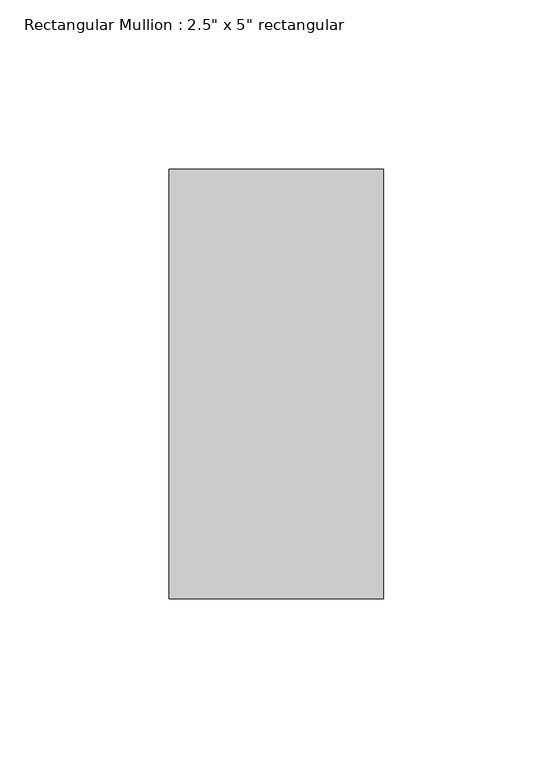
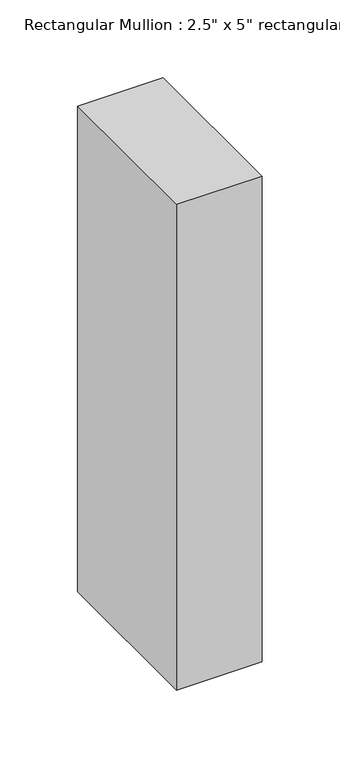
"""IFC4 building model written with IfcOpenShell, lengths in millimetres: member geometry."""

from ifc_helpers import new_model, si_unit, frame, origin, place, context, project, spatial, polyline, outline, extrude, source, transform, mapped, element, save


def member_dfe75557(model_context):
    return source(origin(), model_context, "Body", "SweptSolid", [
        extrude(outline(polyline([(0.0, 63.5), (0.0, -63.5), (-63.5, -63.5), (-63.5, 63.5), (0.0, 63.5)])), frame((0.0, 0.0, -381.0), z_axis=(0.0, 0.0, 1.0), x_axis=(1.0, 0.0, 0.0)), (0.0, 0.0, 1.0), 381.0),
    ])


if __name__ == "__main__":
    model = new_model("IFC4")
    model_context = context("Model", 3, world=origin())
    ifc_project = project(units=[si_unit("LENGTHUNIT", "METRE", prefix="MILLI")], contexts=[model_context])
    site = spatial("IfcSite", under=ifc_project)
    building = spatial("IfcBuilding", under=site)
    placement = place(None, origin())
    member_shape = member_dfe75557(model_context)
    element("IfcMember", 1, ObjectType="Rectangular Mullion : 2.5\" x 5\" rectangular", at=placement, inside=building, context=model_context, shape_type="MappedRepresentation", body=[
        mapped(member_shape, transform((0.0, 0.0, 0.0), x_axis=(1.0, 0.0, 0.0), y_axis=(0.0, 1.0, 0.0), z_axis=(0.0, 0.0, 1.0))),
    ])
    save(model, "model.ifc")

# Revit data of these elements
# Type "Rectangular Mullion : 2.5\" x 5\" rectangular"
#   built-in parameter 1007304 = 0.416667 (stored number, unit not read)
#   built-in parameter 1007301 = 0.104167 (stored number, unit not read)
#   built-in parameter 1007300 = 0.104167 (stored number, unit not read)
# Element 1 (IfcMember, "Rectangular Mullion : 2.5\" x 5\" rectangular")
#   Materials on its faces: "Aluminum"
# Materials
#   "Aluminum": class "Metal", colour RGB 247 247 247, transparency 0, Description = "Aluminum 6061", Cost = 0
